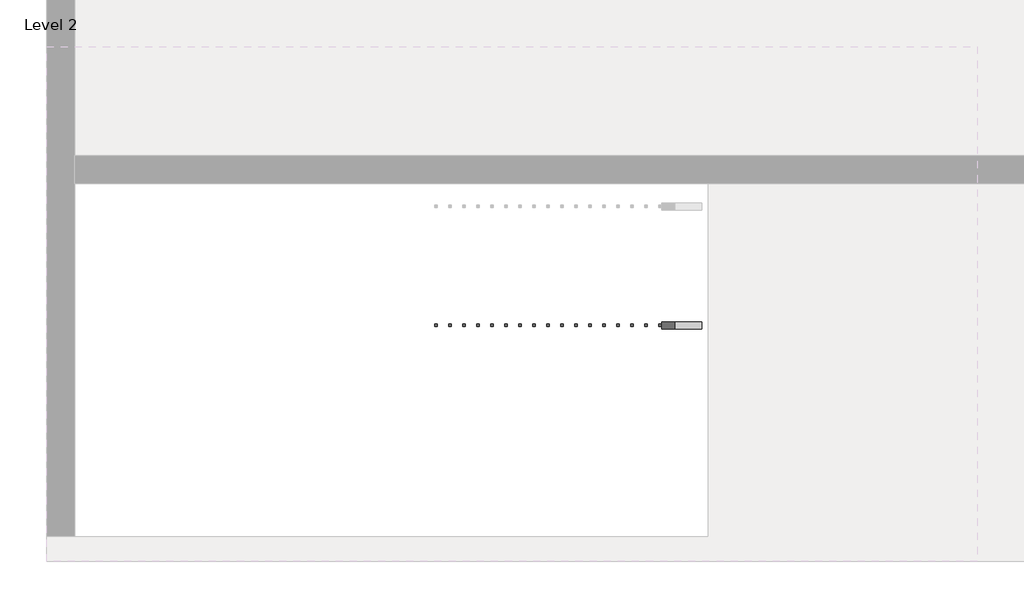
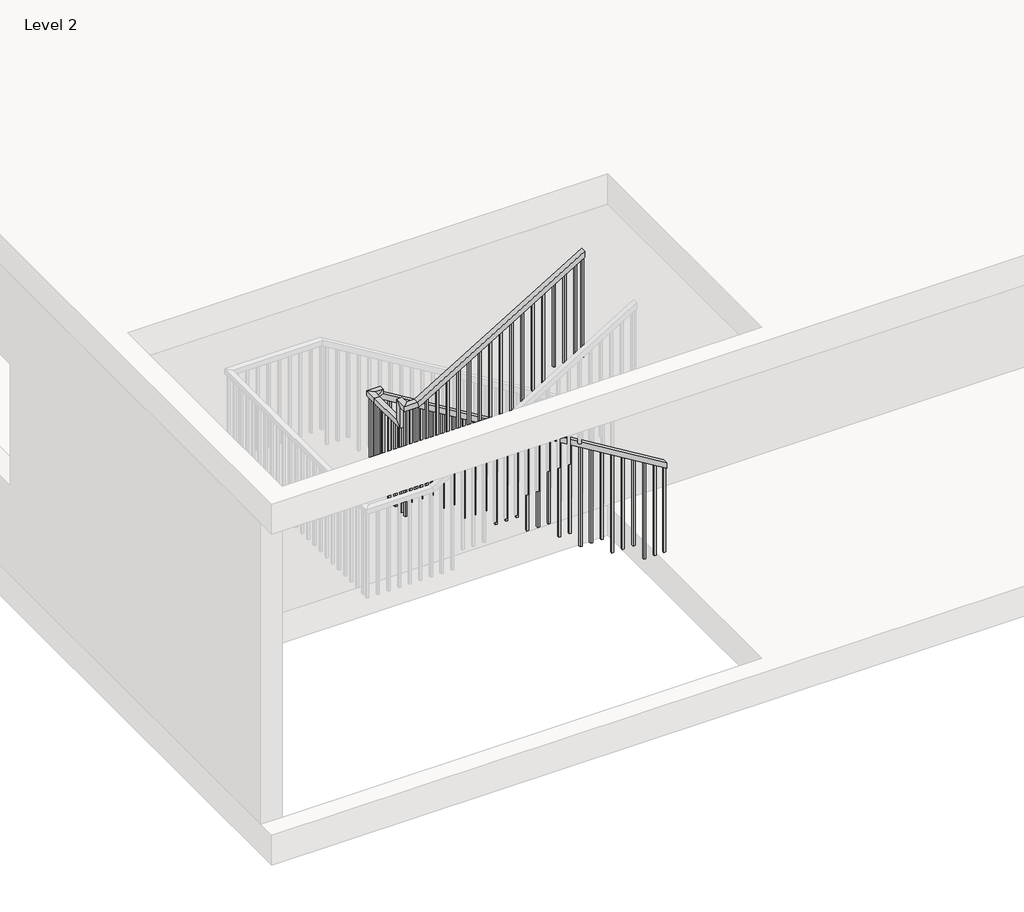
# One storey, part 2 of 2: 1 railing.
"""IFC4 building model written with IfcOpenShell, lengths in millimetres."""

from ifc_helpers import new_model, si_unit, frame, origin, place, context, project, spatial, polyline, outline, extrude, faceted_brep, element, save

model = new_model("IFC4")

# Units and contexts
model_context = context("Model", 3, world=origin())
ifc_project = project(units=[si_unit("LENGTHUNIT", "METRE", prefix="MILLI")], contexts=[model_context])

# Site, building, storey
site = spatial("IfcSite", under=ifc_project)
building = spatial("IfcBuilding", under=site)
storey = spatial("IfcBuildingStorey", under=building, Name="Level 2", Elevation=3048.0)

# Railing
placement = place(None, origin())
element("IfcRailing", 1, ObjectType="Handrail - Rectangular", at=placement, inside=storey, context=model_context, shape_type="SolidModel", body=[
    faceted_brep([(-7036.5382419, -7035.5242744, 4131.7333333), (-7036.5382419, -7035.5242744, 4072.3318731), (-7036.5382419, -6984.7242744, 4072.3318731), (-7036.5382419, -6984.7242744, 4131.7333333), (-9754.3382419, -7035.5242744, 5778.8848485), (-9805.1382419, -7035.5242744, 5750.271267), (-9805.1382419, -6984.7242744, 5750.271267), (-9754.3382419, -6984.7242744, 5778.8848485), (-9830.5382419, -7111.7242744, 5774.2666667), (-9830.5382419, -7111.7242744, 5825.0666667), (-9830.5382419, -7480.6243151, 5825.0666667), (-9830.5382419, -7531.4243151, 5774.2666667), (-9881.3382419, -7111.7242744, 5774.2666667), (-9881.3382419, -7531.4243151, 5774.2666667), (-9881.3382419, -7111.7242744, 5825.0666667), (-9881.3382419, -7480.6243151, 5825.0666667), (-8154.1382419, -7556.8243151, 7010.4), (-8154.1382419, -7607.6243151, 7010.4), (-8154.1382419, -7607.6243151, 6950.9985397), (-8154.1382419, -7556.8243151, 6950.9985397), (-9740.1458325, -7556.8243151, 5989.7818182), (-9754.3382419, -7556.8243151, 6040.5818182), (-9740.1458325, -7607.6243151, 5989.7818182), (-9754.3382419, -7607.6243151, 6040.5818182), (-9830.5382419, -7480.6243151, 6040.5818182), (-9830.5382419, -7531.4243151, 5989.7818182), (-9881.3382419, -7531.4243151, 5989.7818182), (-9881.3382419, -7480.6243151, 6040.5818182), (-9830.5382419, -7556.8243151, 6040.5818182), (-9830.5382419, -7556.8243151, 5989.7818182), (-9881.3382419, -7607.6243151, 5989.7818182), (-9881.3382419, -7607.6243151, 6040.5818182), (-9754.3382419, -7035.5242744, 5825.0666667), (-9805.1382419, -7035.5242744, 5774.2666667), (-9805.1382419, -6984.7242744, 5774.2666667), (-9754.3382419, -6984.7242744, 5825.0666667), (-9830.5382419, -7035.5242744, 5825.0666667), (-9830.5382419, -7035.5242744, 5774.2666667), (-9881.3382419, -6984.7242744, 5774.2666667), (-9881.3382419, -6984.7242744, 5825.0666667)], [[[0, 1, 2, 3]], [[1, 0, 4, 5]], [[2, 1, 5, 6]], [[3, 2, 6, 7]], [[0, 3, 7, 4]], [[8, 9, 10, 11]], [[12, 8, 11, 13]], [[14, 12, 13, 15]], [[9, 14, 15, 10]], [[16, 17, 18, 19]], [[20, 21, 16, 19]], [[22, 20, 19, 18]], [[23, 22, 18, 17]], [[21, 23, 17, 16]], [[11, 10, 24, 25]], [[13, 11, 25, 26]], [[15, 13, 26, 27]], [[10, 15, 27, 24]], [[25, 24, 28, 29]], [[26, 25, 29, 30]], [[27, 26, 30, 31]], [[24, 27, 31, 28]], [[29, 28, 21, 20]], [[30, 29, 20, 22]], [[31, 30, 22, 23]], [[28, 31, 23, 21]], [[5, 4, 32, 33]], [[6, 5, 33, 34]], [[7, 6, 34, 35]], [[4, 7, 35, 32]], [[33, 32, 36, 37]], [[34, 33, 37, 38]], [[35, 34, 38, 39]], [[32, 35, 39, 36]], [[37, 36, 9, 8]], [[38, 37, 8, 12]], [[39, 38, 12, 14]], [[36, 39, 14, 9]]]),
    extrude(outline(polyline([(6899.0439943, -8239.8632419), (5926.6666667, -8239.8632419), (5926.6666667, -8220.8132419), (6910.5894488, -8220.8132419), (6899.0439943, -8239.8632419)])), frame((0.0, -7591.7493151, 0.0), z_axis=(0.0, 1.0, 0.0), x_axis=(0.0, 0.0, 1.0)), (0.0, 0.0, 1.0), 19.05),
    extrude(outline(polyline([(6837.4682367, -8341.4632419), (5926.6666667, -8341.4632419), (5926.6666667, -8322.4132419), (6849.0136913, -8322.4132419), (6837.4682367, -8341.4632419)])), frame((0.0, -7591.7493151, 0.0), z_axis=(0.0, 1.0, 0.0), x_axis=(0.0, 0.0, 1.0)), (0.0, 0.0, 1.0), 19.05),
    extrude(outline(polyline([(6775.8924791, -8443.0632419), (5926.6666667, -8443.0632419), (5926.6666667, -8424.0132419), (6787.4379337, -8424.0132419), (6775.8924791, -8443.0632419)])), frame((0.0, -7591.7493151, 0.0), z_axis=(0.0, 1.0, 0.0), x_axis=(0.0, 0.0, 1.0)), (0.0, 0.0, 1.0), 19.05),
    extrude(outline(polyline([(6714.3167216, -8544.6632419), (5757.3333333, -8544.6632419), (5757.3333333, -8525.6132419), (6725.8621761, -8525.6132419), (6714.3167216, -8544.6632419)])), frame((0.0, -7591.7493151, 0.0), z_axis=(0.0, 1.0, 0.0), x_axis=(0.0, 0.0, 1.0)), (0.0, 0.0, 1.0), 19.05),
    extrude(outline(polyline([(6652.740964, -8646.2632419), (5757.3333333, -8646.2632419), (5757.3333333, -8627.2132419), (6664.2864185, -8627.2132419), (6652.740964, -8646.2632419)])), frame((0.0, -7591.7493151, 0.0), z_axis=(0.0, 1.0, 0.0), x_axis=(0.0, 0.0, 1.0)), (0.0, 0.0, 1.0), 19.05),
    extrude(outline(polyline([(6591.1652064, -8747.8632419), (5588.0, -8747.8632419), (5588.0, -8728.8132419), (6602.710661, -8728.8132419), (6591.1652064, -8747.8632419)])), frame((0.0, -7591.7493151, 0.0), z_axis=(0.0, 1.0, 0.0), x_axis=(0.0, 0.0, 1.0)), (0.0, 0.0, 1.0), 19.05),
    extrude(outline(polyline([(6529.5894488, -8849.4632419), (5588.0, -8849.4632419), (5588.0, -8830.4132419), (6541.1349034, -8830.4132419), (6529.5894488, -8849.4632419)])), frame((0.0, -7591.7493151, 0.0), z_axis=(0.0, 1.0, 0.0), x_axis=(0.0, 0.0, 1.0)), (0.0, 0.0, 1.0), 19.05),
    extrude(outline(polyline([(6468.0136913, -8951.0632419), (5588.0, -8951.0632419), (5588.0, -8932.0132419), (6479.5591458, -8932.0132419), (6468.0136913, -8951.0632419)])), frame((0.0, -7591.7493151, 0.0), z_axis=(0.0, 1.0, 0.0), x_axis=(0.0, 0.0, 1.0)), (0.0, 0.0, 1.0), 19.05),
    extrude(outline(polyline([(6406.4379337, -9052.6632419), (5418.6666667, -9052.6632419), (5418.6666667, -9033.6132419), (6417.9833882, -9033.6132419), (6406.4379337, -9052.6632419)])), frame((0.0, -7591.7493151, 0.0), z_axis=(0.0, 1.0, 0.0), x_axis=(0.0, 0.0, 1.0)), (0.0, 0.0, 1.0), 19.05),
    extrude(outline(polyline([(6344.8621761, -9154.2632419), (5418.6666667, -9154.2632419), (5418.6666667, -9135.2132419), (6356.4076307, -9135.2132419), (6344.8621761, -9154.2632419)])), frame((0.0, -7591.7493151, 0.0), z_axis=(0.0, 1.0, 0.0), x_axis=(0.0, 0.0, 1.0)), (0.0, 0.0, 1.0), 19.05),
    extrude(outline(polyline([(6283.2864185, -9255.8632419), (5418.6666667, -9255.8632419), (5418.6666667, -9236.8132419), (6294.8318731, -9236.8132419), (6283.2864185, -9255.8632419)])), frame((0.0, -7591.7493151, 0.0), z_axis=(0.0, 1.0, 0.0), x_axis=(0.0, 0.0, 1.0)), (0.0, 0.0, 1.0), 19.05),
    extrude(outline(polyline([(6221.710661, -9357.4632419), (5249.3333333, -9357.4632419), (5249.3333333, -9338.4132419), (6233.2561155, -9338.4132419), (6221.710661, -9357.4632419)])), frame((0.0, -7591.7493151, 0.0), z_axis=(0.0, 1.0, 0.0), x_axis=(0.0, 0.0, 1.0)), (0.0, 0.0, 1.0), 19.05),
    extrude(outline(polyline([(6160.1349034, -9459.0632419), (5249.3333333, -9459.0632419), (5249.3333333, -9440.0132419), (6171.6803579, -9440.0132419), (6160.1349034, -9459.0632419)])), frame((0.0, -7591.7493151, 0.0), z_axis=(0.0, 1.0, 0.0), x_axis=(0.0, 0.0, 1.0)), (0.0, 0.0, 1.0), 19.05),
    extrude(outline(polyline([(6098.5591458, -9560.6632419), (5249.3333333, -9560.6632419), (5249.3333333, -9541.6132419), (6110.1046004, -9541.6132419), (6098.5591458, -9560.6632419)])), frame((0.0, -7591.7493151, 0.0), z_axis=(0.0, 1.0, 0.0), x_axis=(0.0, 0.0, 1.0)), (0.0, 0.0, 1.0), 19.05),
    extrude(outline(polyline([(6036.9833882, -9662.2632419), (5080.0, -9662.2632419), (5080.0, -9643.2132419), (6048.5288428, -9643.2132419), (6036.9833882, -9662.2632419)])), frame((0.0, -7591.7493151, 0.0), z_axis=(0.0, 1.0, 0.0), x_axis=(0.0, 0.0, 1.0)), (0.0, 0.0, 1.0), 19.05),
    extrude(outline(polyline([(-9763.8632419, -7572.6993151), (-9744.8132419, -7572.6993151), (-9744.8132419, -7591.7493151), (-9763.8632419, -7591.7493151), (-9763.8632419, -7572.6993151)])), frame((0.0, 0.0, 5080.0), z_axis=(0.0, 0.0, 1.0), x_axis=(1.0, 0.0, 0.0)), (0.0, 0.0, 1.0), 909.7818182),
    extrude(outline(polyline([(-9846.4132419, -7508.5992744), (-9846.4132419, -7527.6492744), (-9865.4632419, -7527.6492744), (-9865.4632419, -7508.5992744), (-9846.4132419, -7508.5992744)])), frame((0.0, 0.0, 4910.6666667), z_axis=(0.0, 0.0, 1.0), x_axis=(1.0, 0.0, 0.0)), (0.0, 0.0, 1.0), 863.6),
    extrude(outline(polyline([(-9846.4132419, -7406.9992744), (-9846.4132419, -7426.0492744), (-9865.4632419, -7426.0492744), (-9865.4632419, -7406.9992744), (-9846.4132419, -7406.9992744)])), frame((0.0, 0.0, 4910.6666667), z_axis=(0.0, 0.0, 1.0), x_axis=(1.0, 0.0, 0.0)), (0.0, 0.0, 1.0), 863.6),
    extrude(outline(polyline([(-9846.4132419, -7305.3992744), (-9846.4132419, -7324.4492744), (-9865.4632419, -7324.4492744), (-9865.4632419, -7305.3992744), (-9846.4132419, -7305.3992744)])), frame((0.0, 0.0, 4910.6666667), z_axis=(0.0, 0.0, 1.0), x_axis=(1.0, 0.0, 0.0)), (0.0, 0.0, 1.0), 863.6),
    extrude(outline(polyline([(-9846.4132419, -7203.7992744), (-9846.4132419, -7222.8492744), (-9865.4632419, -7222.8492744), (-9865.4632419, -7203.7992744), (-9846.4132419, -7203.7992744)])), frame((0.0, 0.0, 4910.6666667), z_axis=(0.0, 0.0, 1.0), x_axis=(1.0, 0.0, 0.0)), (0.0, 0.0, 1.0), 863.6),
    extrude(outline(polyline([(-9846.4132419, -7102.1992744), (-9846.4132419, -7121.2492744), (-9865.4632419, -7121.2492744), (-9865.4632419, -7102.1992744), (-9846.4132419, -7102.1992744)])), frame((0.0, 0.0, 4910.6666667), z_axis=(0.0, 0.0, 1.0), x_axis=(1.0, 0.0, 0.0)), (0.0, 0.0, 1.0), 863.6),
    extrude(outline(polyline([(5740.6500549, -9789.2632419), (4741.3333333, -9789.2632419), (4741.3333333, -9770.2132419), (5729.1046004, -9770.2132419), (5740.6500549, -9789.2632419)])), frame((0.0, -7019.6492744, 0.0), z_axis=(0.0, 1.0, 0.0), x_axis=(0.0, 0.0, 1.0)), (0.0, 0.0, 1.0), 19.05),
    extrude(outline(polyline([(5679.0742973, -9687.6632419), (4741.3333333, -9687.6632419), (4741.3333333, -9668.6132419), (5667.5288428, -9668.6132419), (5679.0742973, -9687.6632419)])), frame((0.0, -7019.6492744, 0.0), z_axis=(0.0, 1.0, 0.0), x_axis=(0.0, 0.0, 1.0)), (0.0, 0.0, 1.0), 19.05),
    extrude(outline(polyline([(5617.4985397, -9586.0632419), (4741.3333333, -9586.0632419), (4741.3333333, -9567.0132419), (5605.9530852, -9567.0132419), (5617.4985397, -9586.0632419)])), frame((0.0, -7019.6492744, 0.0), z_axis=(0.0, 1.0, 0.0), x_axis=(0.0, 0.0, 1.0)), (0.0, 0.0, 1.0), 19.05),
    extrude(outline(polyline([(5555.9227822, -9484.4632419), (4572.0, -9484.4632419), (4572.0, -9465.4132419), (5544.3773276, -9465.4132419), (5555.9227822, -9484.4632419)])), frame((0.0, -7019.6492744, 0.0), z_axis=(0.0, 1.0, 0.0), x_axis=(0.0, 0.0, 1.0)), (0.0, 0.0, 1.0), 19.05),
    extrude(outline(polyline([(5494.3470246, -9382.8632419), (4572.0, -9382.8632419), (4572.0, -9363.8132419), (5482.80157, -9363.8132419), (5494.3470246, -9382.8632419)])), frame((0.0, -7019.6492744, 0.0), z_axis=(0.0, 1.0, 0.0), x_axis=(0.0, 0.0, 1.0)), (0.0, 0.0, 1.0), 19.05),
    extrude(outline(polyline([(5432.771267, -9281.2632419), (4572.0, -9281.2632419), (4572.0, -9262.2132419), (5421.2258125, -9262.2132419), (5432.771267, -9281.2632419)])), frame((0.0, -7019.6492744, 0.0), z_axis=(0.0, 1.0, 0.0), x_axis=(0.0, 0.0, 1.0)), (0.0, 0.0, 1.0), 19.05),
    extrude(outline(polyline([(5371.1955094, -9179.6632419), (4402.6666667, -9179.6632419), (4402.6666667, -9160.6132419), (5359.6500549, -9160.6132419), (5371.1955094, -9179.6632419)])), frame((0.0, -7019.6492744, 0.0), z_axis=(0.0, 1.0, 0.0), x_axis=(0.0, 0.0, 1.0)), (0.0, 0.0, 1.0), 19.05),
    extrude(outline(polyline([(5309.6197519, -9078.0632419), (4402.6666667, -9078.0632419), (4402.6666667, -9059.0132419), (5298.0742973, -9059.0132419), (5309.6197519, -9078.0632419)])), frame((0.0, -7019.6492744, 0.0), z_axis=(0.0, 1.0, 0.0), x_axis=(0.0, 0.0, 1.0)), (0.0, 0.0, 1.0), 19.05),
    extrude(outline(polyline([(5248.0439943, -8976.4632419), (4233.3333333, -8976.4632419), (4233.3333333, -8957.4132419), (5236.4985397, -8957.4132419), (5248.0439943, -8976.4632419)])), frame((0.0, -7019.6492744, 0.0), z_axis=(0.0, 1.0, 0.0), x_axis=(0.0, 0.0, 1.0)), (0.0, 0.0, 1.0), 19.05),
    extrude(outline(polyline([(5186.4682367, -8874.8632419), (4233.3333333, -8874.8632419), (4233.3333333, -8855.8132419), (5174.9227822, -8855.8132419), (5186.4682367, -8874.8632419)])), frame((0.0, -7019.6492744, 0.0), z_axis=(0.0, 1.0, 0.0), x_axis=(0.0, 0.0, 1.0)), (0.0, 0.0, 1.0), 19.05),
    extrude(outline(polyline([(5124.8924791, -8773.2632419), (4233.3333333, -8773.2632419), (4233.3333333, -8754.2132419), (5113.3470246, -8754.2132419), (5124.8924791, -8773.2632419)])), frame((0.0, -7019.6492744, 0.0), z_axis=(0.0, 1.0, 0.0), x_axis=(0.0, 0.0, 1.0)), (0.0, 0.0, 1.0), 19.05),
    extrude(outline(polyline([(5063.3167216, -8671.6632419), (4064.0, -8671.6632419), (4064.0, -8652.6132419), (5051.771267, -8652.6132419), (5063.3167216, -8671.6632419)])), frame((0.0, -7019.6492744, 0.0), z_axis=(0.0, 1.0, 0.0), x_axis=(0.0, 0.0, 1.0)), (0.0, 0.0, 1.0), 19.05),
    extrude(outline(polyline([(5001.740964, -8570.0632419), (4064.0, -8570.0632419), (4064.0, -8551.0132419), (4990.1955094, -8551.0132419), (5001.740964, -8570.0632419)])), frame((0.0, -7019.6492744, 0.0), z_axis=(0.0, 1.0, 0.0), x_axis=(0.0, 0.0, 1.0)), (0.0, 0.0, 1.0), 19.05),
    extrude(outline(polyline([(4940.1652064, -8468.4632419), (4064.0, -8468.4632419), (4064.0, -8449.4132419), (4928.6197519, -8449.4132419), (4940.1652064, -8468.4632419)])), frame((0.0, -7019.6492744, 0.0), z_axis=(0.0, 1.0, 0.0), x_axis=(0.0, 0.0, 1.0)), (0.0, 0.0, 1.0), 19.05),
    extrude(outline(polyline([(4878.5894488, -8366.8632419), (3894.6666667, -8366.8632419), (3894.6666667, -8347.8132419), (4867.0439943, -8347.8132419), (4878.5894488, -8366.8632419)])), frame((0.0, -7019.6492744, 0.0), z_axis=(0.0, 1.0, 0.0), x_axis=(0.0, 0.0, 1.0)), (0.0, 0.0, 1.0), 19.05),
    extrude(outline(polyline([(4817.0136913, -8265.2632419), (3894.6666667, -8265.2632419), (3894.6666667, -8246.2132419), (4805.4682367, -8246.2132419), (4817.0136913, -8265.2632419)])), frame((0.0, -7019.6492744, 0.0), z_axis=(0.0, 1.0, 0.0), x_axis=(0.0, 0.0, 1.0)), (0.0, 0.0, 1.0), 19.05),
    extrude(outline(polyline([(4755.4379337, -8163.6632419), (3894.6666667, -8163.6632419), (3894.6666667, -8144.6132419), (4743.8924791, -8144.6132419), (4755.4379337, -8163.6632419)])), frame((0.0, -7019.6492744, 0.0), z_axis=(0.0, 1.0, 0.0), x_axis=(0.0, 0.0, 1.0)), (0.0, 0.0, 1.0), 19.05),
    extrude(outline(polyline([(4693.8621761, -8062.0632419), (3725.3333333, -8062.0632419), (3725.3333333, -8043.0132419), (4682.3167216, -8043.0132419), (4693.8621761, -8062.0632419)])), frame((0.0, -7019.6492744, 0.0), z_axis=(0.0, 1.0, 0.0), x_axis=(0.0, 0.0, 1.0)), (0.0, 0.0, 1.0), 19.05),
    extrude(outline(polyline([(4632.2864185, -7960.4632419), (3725.3333333, -7960.4632419), (3725.3333333, -7941.4132419), (4620.740964, -7941.4132419), (4632.2864185, -7960.4632419)])), frame((0.0, -7019.6492744, 0.0), z_axis=(0.0, 1.0, 0.0), x_axis=(0.0, 0.0, 1.0)), (0.0, 0.0, 1.0), 19.05),
    extrude(outline(polyline([(4570.710661, -7858.8632419), (3556.0, -7858.8632419), (3556.0, -7839.8132419), (4559.1652064, -7839.8132419), (4570.710661, -7858.8632419)])), frame((0.0, -7019.6492744, 0.0), z_axis=(0.0, 1.0, 0.0), x_axis=(0.0, 0.0, 1.0)), (0.0, 0.0, 1.0), 19.05),
    extrude(outline(polyline([(4509.1349034, -7757.2632419), (3556.0, -7757.2632419), (3556.0, -7738.2132419), (4497.5894488, -7738.2132419), (4509.1349034, -7757.2632419)])), frame((0.0, -7019.6492744, 0.0), z_axis=(0.0, 1.0, 0.0), x_axis=(0.0, 0.0, 1.0)), (0.0, 0.0, 1.0), 19.05),
    extrude(outline(polyline([(4447.5591458, -7655.6632419), (3556.0, -7655.6632419), (3556.0, -7636.6132419), (4436.0136913, -7636.6132419), (4447.5591458, -7655.6632419)])), frame((0.0, -7019.6492744, 0.0), z_axis=(0.0, 1.0, 0.0), x_axis=(0.0, 0.0, 1.0)), (0.0, 0.0, 1.0), 19.05),
    extrude(outline(polyline([(4385.9833882, -7554.0632419), (3386.6666667, -7554.0632419), (3386.6666667, -7535.0132419), (4374.4379337, -7535.0132419), (4385.9833882, -7554.0632419)])), frame((0.0, -7019.6492744, 0.0), z_axis=(0.0, 1.0, 0.0), x_axis=(0.0, 0.0, 1.0)), (0.0, 0.0, 1.0), 19.05),
    extrude(outline(polyline([(4324.4076307, -7452.4632419), (3386.6666667, -7452.4632419), (3386.6666667, -7433.4132419), (4312.8621761, -7433.4132419), (4324.4076307, -7452.4632419)])), frame((0.0, -7019.6492744, 0.0), z_axis=(0.0, 1.0, 0.0), x_axis=(0.0, 0.0, 1.0)), (0.0, 0.0, 1.0), 19.05),
    extrude(outline(polyline([(4262.8318731, -7350.8632419), (3386.6666667, -7350.8632419), (3386.6666667, -7331.8132419), (4251.2864185, -7331.8132419), (4262.8318731, -7350.8632419)])), frame((0.0, -7019.6492744, 0.0), z_axis=(0.0, 1.0, 0.0), x_axis=(0.0, 0.0, 1.0)), (0.0, 0.0, 1.0), 19.05),
    extrude(outline(polyline([(4201.2561155, -7249.2632419), (3217.3333333, -7249.2632419), (3217.3333333, -7230.2132419), (4189.710661, -7230.2132419), (4201.2561155, -7249.2632419)])), frame((0.0, -7019.6492744, 0.0), z_axis=(0.0, 1.0, 0.0), x_axis=(0.0, 0.0, 1.0)), (0.0, 0.0, 1.0), 19.05),
    extrude(outline(polyline([(4139.6803579, -7147.6632419), (3217.3333333, -7147.6632419), (3217.3333333, -7128.6132419), (4128.1349034, -7128.6132419), (4139.6803579, -7147.6632419)])), frame((0.0, -7019.6492744, 0.0), z_axis=(0.0, 1.0, 0.0), x_axis=(0.0, 0.0, 1.0)), (0.0, 0.0, 1.0), 19.05),
    extrude(outline(polyline([(-9865.4632419, -7572.6993151), (-9846.4132419, -7572.6993151), (-9846.4132419, -7591.7493151), (-9865.4632419, -7591.7493151), (-9865.4632419, -7572.6993151)])), frame((0.0, 0.0, 4910.6666667), z_axis=(0.0, 0.0, 1.0), x_axis=(1.0, 0.0, 0.0)), (0.0, 0.0, 1.0), 1079.1151515),
    extrude(outline(polyline([(-9846.4132419, -7019.6492744), (-9865.4632419, -7019.6492744), (-9865.4632419, -7000.5992744), (-9846.4132419, -7000.5992744), (-9846.4132419, -7019.6492744)])), frame((0.0, 0.0, 4910.6666667), z_axis=(0.0, 0.0, 1.0), x_axis=(1.0, 0.0, 0.0)), (0.0, 0.0, 1.0), 863.6),
    extrude(outline(polyline([(-9821.0132419, -7019.6492744), (-9840.0632419, -7019.6492744), (-9840.0632419, -7000.5992744), (-9821.0132419, -7000.5992744), (-9821.0132419, -7019.6492744)])), frame((0.0, 0.0, 4910.6666667), z_axis=(0.0, 0.0, 1.0), x_axis=(1.0, 0.0, 0.0)), (0.0, 0.0, 1.0), 863.6),
    extrude(outline(polyline([(6939.4530852, -8173.1882419), (5926.6666667, -8173.1882419), (5926.6666667, -8154.1382419), (6950.9985397, -8154.1382419), (6939.4530852, -8173.1882419)])), frame((0.0, -7591.7493151, 0.0), z_axis=(0.0, 1.0, 0.0), x_axis=(0.0, 0.0, 1.0)), (0.0, 0.0, 1.0), 19.05),
    extrude(outline(polyline([(4083.8773276, -7055.5882419), (3217.3333333, -7055.5882419), (3217.3333333, -7036.5382419), (4072.3318731, -7036.5382419), (4083.8773276, -7055.5882419)])), frame((0.0, -7019.6492744, 0.0), z_axis=(0.0, 1.0, 0.0), x_axis=(0.0, 0.0, 1.0)), (0.0, 0.0, 1.0), 19.05),
])

save(model, "model.ifc")

# Revit data of these elements
# Type "Handrail - Rectangular"
#   Assembly Code = "C2010400"
#   built-in parameter 1008612 = 0.0416667 (stored number, unit not read)
#   built-in parameter 1008611 = 0.0416667 (stored number, unit not read)
#   built-in parameter 1008609 = 0.333333 (stored number, unit not read)
#   built-in parameter 1008604 = 0.166667 (stored number, unit not read)
#   built-in parameter 1008603 = 0.166667 (stored number, unit not read)
#   Railing Height = 3' - 0"
#   built-in parameter 1008630 = 2
#   built-in parameter 1008610 = 2
#   built-in parameter 1008618 = Baluster - Square : 3/4"
# Element 1 (IfcRailing, "Handrail - Rectangular")
#   Phase Created = New Construction
